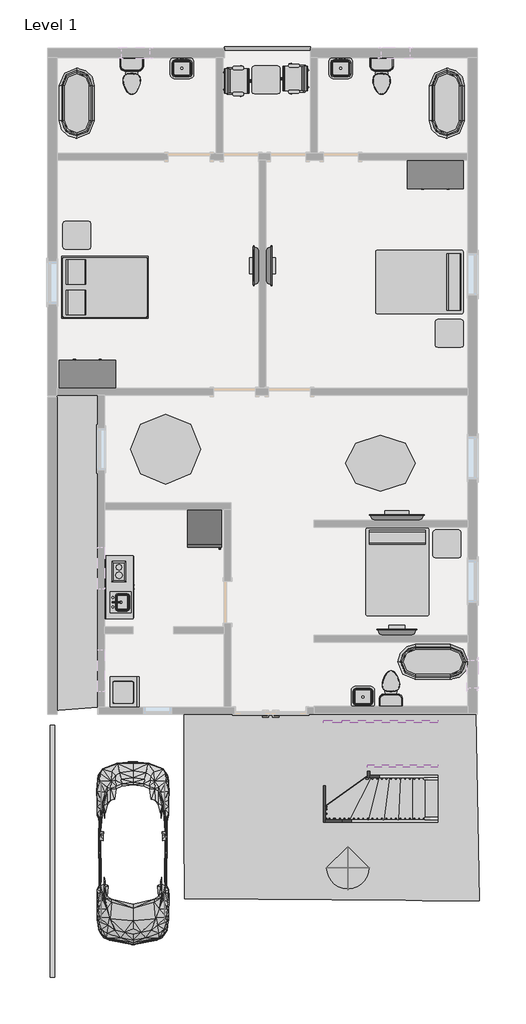
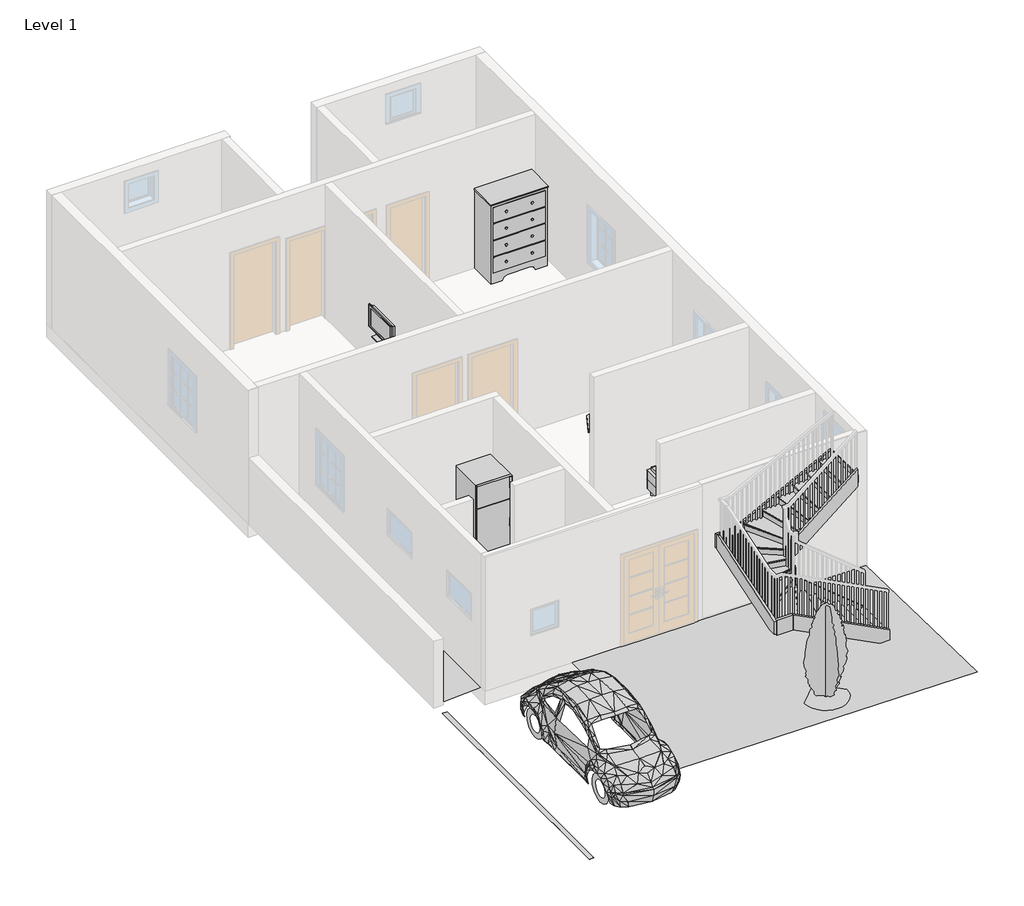
# One storey, part 3 of 3: 18 furniture elements, 10 flow terminals, 8 members, 8 proxies, 1 geographic element, 1 railing, 1 stair flight.
"""IFC4 building model written with IfcOpenShell, lengths in millimetres."""

from ifc_helpers import new_model, si_unit, point, frame, origin, origin_with_axes, place, context, project, spatial, polyline, ellipse_curve, trimmed, outline, extrude, triangles, transform, mapped, element, save
from ifc_brep_helpers import plane_surface, extruded_surface, advanced_brep
from components import proxy_fe84b772, proxy_844211aa, parking_space_9_x_18_90_deg_b8b21359, rpc_beetle_rpc_beetle_3ce7ba48, proxy_a13a33b2, proxy_718fa39f, flow_terminal_871c2e40, flow_terminal_62a433f7, toilet_domestic_3d_toilet_domestic_3d_f7549cf7, toilet_domestic_3d_toilet_domestic_3d_183bbd19, flow_terminal_b374fae2, furniture_c8abb964, furniture_0253826f, chair_task_arms_chair_task_arms_fa5a08ef, furniture_95afb093, furniture_9fa109b2, furniture_56245f3a, furniture_d9bcc661, furniture_bbcc68ce, furniture_743965d2, furniture_bcf351fa, rpc_tree_conifer_0001_chinese_juniper_7_1b9786cd, stair_flight_62da4333

model = new_model("IFC4")

# Units and contexts
model_context = context("Model", 3, world=origin())
ifc_project = project(units=[si_unit("LENGTHUNIT", "METRE", prefix="MILLI")], contexts=[model_context])

# Site, building, storey
site = spatial("IfcSite", under=ifc_project)
building = spatial("IfcBuilding", under=site)
storey = spatial("IfcBuildingStorey", under=building, Name="Level 1", Elevation=0.0)

# Proxies
placement = place(None, origin())
element("IfcBuildingElementProxy", 1, Name="Building Element Proxy", at=placement, inside=storey, context=model_context, shape_type="Tessellation", body=[
    triangles([(-8788.6245987, -108.0463665, 0.0), (-8767.5415833, -4098.269323, 0.0), (-2526.9445953, -4159.926606, 0.0), (-2604.3049896, -82.6463725, 0.0), (-8917.3917389, -4057.5674469, 0.0), (-8941.0245987, -2597.2464088, 0.0), (-8941.0245987, -108.0463665, 0.0), (-8936.3004684, -4107.611776, 0.0)], [[8, 5, 6], [5, 8, 2], [1, 7, 6], [6, 5, 2], [3, 4, 6], [3, 2, 8], [1, 4, 7], [1, 6, 4], [6, 2, 3]], closed=False),
])
element("IfcBuildingElementProxy", 2, Name="Building Element Proxy", at=placement, inside=storey, context=model_context, shape_type="Tessellation", body=[
    triangles([(-11709.6247925, 6826.153688, 0.0), (-10820.6244049, 6826.153688, 0.0), (-10820.6244049, 44.353629, 0.0), (-11811.2244049, -31.846371, 0.0)], [[1, 4, 3], [3, 2, 1]], closed=False),
])
proxy_shape = proxy_fe84b772(model_context)
element("IfcBuildingElementProxy", 3, Name="Cook Top-2 Unit : 12\" x 18\"", ObjectType="Cook Top-2 Unit : 12\" x 18\"", at=placement, inside=storey, context=model_context, shape_type="MappedRepresentation", body=[
    mapped(proxy_shape, transform((-10287.2247577, 3033.3661295, 0.0), x_axis=(-1.0, 0.0, 0.0), y_axis=(0.0, -1.0, 0.0), z_axis=(0.0, 0.0, 1.0))),
])
proxy_2_shape = proxy_844211aa(model_context)
element("IfcBuildingElementProxy", 4, Name="Kitchenette - Small : 54\"", ObjectType="Kitchenette - Small : 54\"", at=placement, inside=storey, context=model_context, shape_type="MappedRepresentation", body=[
    mapped(proxy_2_shape, transform((-10668.2247577, 2641.503629, 0.0), x_axis=(0.0, 1.0, 0.0), y_axis=(-1.0, 0.0, 0.0), z_axis=(0.0, 0.0, 1.0))),
])
parking_space_9_x_18_90_deg_shape = parking_space_9_x_18_90_deg_b8b21359(model_context)
element("IfcBuildingElementProxy", 5, Name="Parking Space : 9' x 18' - 90 deg", ObjectType="Parking Space : 9' x 18' - 90 deg", at=placement, inside=storey, context=model_context, shape_type="MappedRepresentation", body=[
    mapped(parking_space_9_x_18_90_deg_shape, transform((-11811.2247577, -336.646371, 0.0), x_axis=(1.0, 0.0, 0.0), y_axis=(0.0, 1.0, 0.0), z_axis=(0.0, 0.0, 1.0))),
])
rpc_beetle_rpc_beetle_shape = rpc_beetle_rpc_beetle_3ce7ba48(model_context)
element("IfcBuildingElementProxy", 6, Name="RPC Beetle : RPC Beetle", ObjectType="RPC Beetle : RPC Beetle", at=placement, inside=storey, context=model_context, shape_type="MappedRepresentation", body=[
    mapped(rpc_beetle_rpc_beetle_shape, transform((-10058.6247577, -1886.046371, 0.0), x_axis=(-1.0000000000000004, 0.0, 0.0), y_axis=(0.0, -1.0000000000000004, 0.0), z_axis=(0.0, 0.0, 1.0))),
])
proxy_3_shape = proxy_a13a33b2(model_context)
element("IfcBuildingElementProxy", 7, Name="Refrigerator : 30\" x 32\" RH", ObjectType="Refrigerator : 30\" x 32\" RH", at=placement, inside=storey, context=model_context, shape_type="MappedRepresentation", body=[
    mapped(proxy_3_shape, transform((-8501.2872577, 3948.4046575, 0.0), x_axis=(1.0, 0.0, 0.0), y_axis=(0.0, 1.0, 0.0), z_axis=(0.0, 0.0, 1.0))),
])
proxy_4_shape = proxy_718fa39f(model_context)
element("IfcBuildingElementProxy", 8, Name="Washer : 27\" x 25\" x 35\"", ObjectType="Washer : 27\" x 25\" x 35\"", at=placement, inside=storey, context=model_context, shape_type="MappedRepresentation", body=[
    mapped(proxy_4_shape, transform((-10515.8247577, 793.9040642, 0.0), x_axis=(0.0, -1.0000000000000016, 0.0), y_axis=(1.0000000000000016, 0.0, 0.0), z_axis=(0.0, 0.0, 1.0))),
])

# Flow terminals
flow_terminal_shape = flow_terminal_871c2e40(model_context)
element("IfcFlowTerminal", 9, ObjectType="Sink Kitchen-Island : 18\" x 18\"", at=placement, inside=storey, context=model_context, shape_type="MappedRepresentation", body=[
    mapped(flow_terminal_shape, transform((-10322.9793566, 2314.3520934, 0.0), x_axis=(0.0, 1.0, 0.0), y_axis=(-1.0, 0.0, 0.0), z_axis=(0.0, 0.0, 1.0))),
])
flow_terminal_2_shape = flow_terminal_62a433f7(model_context)
element("IfcFlowTerminal", 10, ObjectType="Sink Vanity-Square : 20\" x 18\"", at=placement, inside=storey, context=model_context, shape_type="MappedRepresentation", body=[
    mapped(flow_terminal_2_shape, transform((-9007.5139982, 13986.6082279, 304.8), x_axis=(1.0, 0.0, 0.0), y_axis=(0.0, 1.0, 0.0), z_axis=(0.0, 0.0, 1.0))),
])
element("IfcFlowTerminal", 11, ObjectType="Sink Vanity-Square : 20\" x 18\"", at=placement, inside=storey, context=model_context, shape_type="MappedRepresentation", body=[
    mapped(flow_terminal_2_shape, transform((-5553.1139982, 13986.6082279, 304.8), x_axis=(1.0, 0.0, 0.0), y_axis=(0.0, 1.0, 0.0), z_axis=(0.0, 0.0, 1.0))),
])
element("IfcFlowTerminal", 12, ObjectType="Sink Vanity-Square : 20\" x 18\"", at=placement, inside=storey, context=model_context, shape_type="MappedRepresentation", body=[
    mapped(flow_terminal_2_shape, transform((-5039.1355171, 224.4990301, 304.8), x_axis=(-1.0, 0.0, 0.0), y_axis=(0.0, -1.0, 0.0), z_axis=(0.0, 0.0, 1.0))),
])
toilet_domestic_3d_toilet_domestic_3d_shape = toilet_domestic_3d_toilet_domestic_3d_f7549cf7(model_context)
toilet_domestic_3d_toilet_domestic_3d_2_shape = toilet_domestic_3d_toilet_domestic_3d_183bbd19(model_context)
element("IfcFlowTerminal", 13, ObjectType="Toilet-Domestic-3D : Toilet-Domestic-3D", at=placement, inside=storey, context=model_context, shape_type="MappedRepresentation", body=[
    mapped(toilet_domestic_3d_toilet_domestic_3d_shape, transform((-10084.0247577, 13672.0576017, 0.0), x_axis=(1.0, 0.0, 0.0), y_axis=(0.0, 1.0, 0.0), z_axis=(0.0, 0.0, 1.0))),
    mapped(toilet_domestic_3d_toilet_domestic_3d_2_shape, transform((-10084.0247577, 13672.0576017, 0.0), x_axis=(1.0, 0.0, 0.0), y_axis=(0.0, 1.0, 0.0), z_axis=(0.0, 0.0, 1.0))),
])
element("IfcFlowTerminal", 14, ObjectType="Toilet-Domestic-3D : Toilet-Domestic-3D", at=placement, inside=storey, context=model_context, shape_type="MappedRepresentation", body=[
    mapped(toilet_domestic_3d_toilet_domestic_3d_shape, transform((-4648.4247577, 13672.0576017, 0.0), x_axis=(1.0, 0.0, 0.0), y_axis=(0.0, 1.0, 0.0), z_axis=(0.0, 0.0, 1.0))),
    mapped(toilet_domestic_3d_toilet_domestic_3d_2_shape, transform((-4648.4247577, 13672.0576017, 0.0), x_axis=(1.0, 0.0, 0.0), y_axis=(0.0, 1.0, 0.0), z_axis=(0.0, 0.0, 1.0))),
])
element("IfcFlowTerminal", 15, ObjectType="Toilet-Domestic-3D : Toilet-Domestic-3D", at=placement, inside=storey, context=model_context, shape_type="MappedRepresentation", body=[
    mapped(toilet_domestic_3d_toilet_domestic_3d_shape, transform((-4445.2247577, 539.0496564, 0.0), x_axis=(-1.0000000000000002, 0.0, 0.0), y_axis=(0.0, -1.0000000000000002, 0.0), z_axis=(0.0, 0.0, 1.0))),
    mapped(toilet_domestic_3d_toilet_domestic_3d_2_shape, transform((-4445.2247577, 539.0496564, 0.0), x_axis=(-1.0000000000000002, 0.0, 0.0), y_axis=(0.0, -1.0000000000000002, 0.0), z_axis=(0.0, 0.0, 1.0))),
])
flow_terminal_3_shape = flow_terminal_b374fae2(model_context)
element("IfcFlowTerminal", 16, ObjectType="Tub-Free Standing-3D : 30\" x 60\"", at=placement, inside=storey, context=model_context, shape_type="MappedRepresentation", body=[
    mapped(flow_terminal_3_shape, transform((-11277.8247577, 13176.153629, 0.0), x_axis=(1.0, 0.0, 0.0), y_axis=(0.0, 1.0, 0.0), z_axis=(0.0, 0.0, 1.0))),
])
element("IfcFlowTerminal", 17, ObjectType="Tub-Free Standing-3D : 30\" x 60\"", at=placement, inside=storey, context=model_context, shape_type="MappedRepresentation", body=[
    mapped(flow_terminal_3_shape, transform((-3226.0247577, 13176.153629, 0.0), x_axis=(1.0, 0.0, 0.0), y_axis=(0.0, 1.0, 0.0), z_axis=(0.0, 0.0, 1.0))),
])
element("IfcFlowTerminal", 18, ObjectType="Tub-Free Standing-3D : 30\" x 60\"", at=placement, inside=storey, context=model_context, shape_type="MappedRepresentation", body=[
    mapped(flow_terminal_3_shape, transform((-3530.8247577, 1034.953629, 0.0), x_axis=(0.0, -1.0000000000000004, 0.0), y_axis=(1.0000000000000004, 0.0, 0.0), z_axis=(0.0, 0.0, 1.0))),
])

# Furniture
furniture_shape = furniture_c8abb964(model_context)
element("IfcFurniture", 19, ObjectType="Bed-Box : Double 53\" x 74\"", at=placement, inside=storey, context=model_context, shape_type="MappedRepresentation", body=[
    mapped(furniture_shape, transform((-10902.6542659, 8836.50117, 0.0), x_axis=(0.0, 1.0000000000000002, 0.0), y_axis=(-1.0000000000000002, 0.0, 0.0), z_axis=(0.0, 0.0, 1.0))),
])
furniture_2_shape = furniture_0253826f(model_context)
element("IfcFurniture", 20, ObjectType="Bed-Standard.0001 : Double 54\" x 75\"", at=placement, inside=storey, context=model_context, shape_type="MappedRepresentation", body=[
    mapped(furniture_2_shape, transform((-3777.3296757, 9561.4421536, 0.0), x_axis=(0.0, -1.0000000000000002, 0.0), y_axis=(1.0000000000000002, 0.0, 0.0), z_axis=(0.0, 0.0, 1.0))),
])
element("IfcFurniture", 21, ObjectType="Bed-Standard.0001 : Double 54\" x 75\"", at=placement, inside=storey, context=model_context, shape_type="MappedRepresentation", body=[
    mapped(furniture_2_shape, transform((-4577.0132823, 3036.348711, 0.0), x_axis=(1.0000000000000004, 0.0, 0.0), y_axis=(0.0, 1.0000000000000004, 0.0), z_axis=(0.0, 0.0, 1.0))),
])
chair_task_arms_chair_task_arms_shape = chair_task_arms_chair_task_arms_fa5a08ef(model_context)
element("IfcFurniture", 22, ObjectType="Chair-Task Arms : Chair-Task Arms", at=placement, inside=storey, context=model_context, shape_type="MappedRepresentation", body=[
    mapped(chair_task_arms_chair_task_arms_shape, transform((-6509.078856, 13568.5628094, 0.0), x_axis=(0.0, 1.0000000000000009, 0.0), y_axis=(-1.0000000000000009, 0.0, 0.0), z_axis=(0.0, 0.0, 1.0))),
])
element("IfcFurniture", 23, ObjectType="Chair-Task Arms : Chair-Task Arms", at=placement, inside=storey, context=model_context, shape_type="MappedRepresentation", body=[
    mapped(chair_task_arms_chair_task_arms_shape, transform((-7816.9706593, 13799.7444487, 0.0), x_axis=(0.0, -1.0000000000000004, 0.0), y_axis=(1.0000000000000004, 0.0, 0.0), z_axis=(0.0, 0.0, 1.0))),
])
furniture_3_shape = furniture_95afb093(model_context)
element("IfcFurniture", 24, ObjectType="Counter Top w Sink Hole : 24\" Depth", at=placement, inside=storey, context=model_context, shape_type="MappedRepresentation", body=[
    mapped(furniture_3_shape, transform((-10668.2247577, 3174.903629, 0.0), x_axis=(0.0, 1.0, 0.0), y_axis=(-1.0, 0.0, 0.0), z_axis=(0.0, 0.0, 1.0))),
])
furniture_4_shape = furniture_9fa109b2(model_context)
element("IfcFurniture", 25, ObjectType="Dresser : 48\" x 72\" x 24\"", at=placement, inside=storey, context=model_context, shape_type="MappedRepresentation", body=[
    mapped(furniture_4_shape, transform((-11318.4180175, 6920.1906749, 0.0), x_axis=(-1.0000000000000004, 0.0, 0.0), y_axis=(0.0, -1.0000000000000004, 0.0), z_axis=(0.0, 0.0, 1.0))),
])
element("IfcFurniture", 26, ObjectType="Dresser : 48\" x 72\" x 24\"", at=placement, inside=storey, context=model_context, shape_type="MappedRepresentation", body=[
    mapped(furniture_4_shape, transform((-3210.8314978, 11989.9165831, 0.0), x_axis=(1.0, 0.0, 0.0), y_axis=(0.0, 1.0, 0.0), z_axis=(0.0, 0.0, 1.0))),
])
furniture_5_shape = furniture_56245f3a(model_context)
element("IfcFurniture", 27, ObjectType="TV - Flat Screen : 32\"", at=placement, inside=storey, context=model_context, shape_type="MappedRepresentation", body=[
    mapped(furniture_5_shape, transform((-7373.9633813, 9641.6091149, 914.4), x_axis=(0.0, -1.0000000000000004, 0.0), y_axis=(1.0000000000000004, 0.0, 0.0), z_axis=(0.0, 0.0, 1.0))),
])
element("IfcFurniture", 28, ObjectType="TV - Flat Screen : 32\"", at=placement, inside=storey, context=model_context, shape_type="MappedRepresentation", body=[
    mapped(furniture_5_shape, transform((-7104.486134, 9649.4981432, 914.4), x_axis=(0.0, 1.0000000000000002, 0.0), y_axis=(-1.0000000000000002, 0.0, 0.0), z_axis=(0.0, 0.0, 1.0))),
])
element("IfcFurniture", 29, ObjectType="TV - Flat Screen : 32\"", at=placement, inside=storey, context=model_context, shape_type="MappedRepresentation", body=[
    mapped(furniture_5_shape, transform((-4322.1692718, 1677.6922527, 914.4), x_axis=(-1.0000000000000002, 0.0, 0.0), y_axis=(0.0, -1.0000000000000002, 0.0), z_axis=(0.0, 0.0, 1.0))),
])
furniture_6_shape = furniture_d9bcc661(model_context)
element("IfcFurniture", 30, ObjectType="TV - Flat Screen : 46\"", at=placement, inside=storey, context=model_context, shape_type="MappedRepresentation", body=[
    mapped(furniture_6_shape, transform((-4322.1692718, 4166.8922527, 914.4), x_axis=(-0.9999999999999998, 0.0, 0.0), y_axis=(0.0, -0.9999999999999998, 0.0), z_axis=(0.0, 0.0, 1.0))),
])
furniture_7_shape = furniture_bbcc68ce(model_context)
element("IfcFurniture", 31, ObjectType="Table-Dining Round w Chairs : 60\" Diameter", at=placement, inside=storey, context=model_context, shape_type="MappedRepresentation", body=[
    mapped(furniture_7_shape, transform((-9451.1067249, 5842.6323176, 0.0), x_axis=(1.0, 0.0, 0.0), y_axis=(0.0, 1.0, 0.0), z_axis=(0.0, 0.0, 1.0))),
])
furniture_8_shape = furniture_743965d2(model_context)
element("IfcFurniture", 32, ObjectType="Table-Ellipse : 60\" x 48\"", at=placement, inside=storey, context=model_context, shape_type="MappedRepresentation", body=[
    mapped(furniture_8_shape, transform((-4673.8247577, 5352.953629, 0.0), x_axis=(1.0, 0.0, 0.0), y_axis=(0.0, 1.0, 0.0), z_axis=(0.0, 0.0, 1.0))),
])
furniture_9_shape = furniture_bcf351fa(model_context)
element("IfcFurniture", 33, ObjectType="Table-End : 24\" x 24\"", at=placement, inside=storey, context=model_context, shape_type="MappedRepresentation", body=[
    mapped(furniture_9_shape, transform((-11586.358388, 10153.553629, 0.0), x_axis=(1.0, 0.0, 0.0), y_axis=(0.0, 1.0, 0.0), z_axis=(0.0, 0.0, 1.0))),
])
element("IfcFurniture", 34, ObjectType="Table-End : 24\" x 24\"", at=placement, inside=storey, context=model_context, shape_type="MappedRepresentation", body=[
    mapped(furniture_9_shape, transform((-3483.758388, 8019.953629, 0.0), x_axis=(1.0, 0.0, 0.0), y_axis=(0.0, 1.0, 0.0), z_axis=(0.0, 0.0, 1.0))),
])
element("IfcFurniture", 35, ObjectType="Table-End : 24\" x 24\"", at=placement, inside=storey, context=model_context, shape_type="MappedRepresentation", body=[
    mapped(furniture_9_shape, transform((-7471.558388, 13531.753629, 0.0), x_axis=(1.0, 0.0, 0.0), y_axis=(0.0, 1.0, 0.0), z_axis=(0.0, 0.0, 1.0))),
])
element("IfcFurniture", 36, ObjectType="Table-End : 24\" x 24\"", at=placement, inside=storey, context=model_context, shape_type="MappedRepresentation", body=[
    mapped(furniture_9_shape, transform((-3534.558388, 3447.953629, 0.0), x_axis=(1.0, 0.0, 0.0), y_axis=(0.0, 1.0, 0.0), z_axis=(0.0, 0.0, 1.0))),
])

# Geographic element
rpc_tree_conifer_0001_chinese_juniper_7_shape = rpc_tree_conifer_0001_chinese_juniper_7_1b9786cd(model_context)
element("IfcGeographicElement", 37, ObjectType="RPC Tree - Conifer.0001 : Chinese Juniper - 7'", at=placement, inside=storey, context=model_context, shape_type="MappedRepresentation", body=[
    mapped(rpc_tree_conifer_0001_chinese_juniper_7_shape, transform((-5385.2214287, -3435.446371, 0.0), x_axis=(1.0, 0.0, 0.0), y_axis=(0.0, 1.0, 0.0), z_axis=(0.0, 0.0, 1.0))),
])

# Members
element("IfcMember", 38, ObjectType="Stringer - 2\" Width", at=placement, inside=storey, context=model_context, shape_type="SweptSolid", body=[
    extrude(outline(polyline([(0.0, -3425.4930658), (229.639954, -3425.4930658), (1305.3956453, -5512.9102575), (962.500629, -5512.9102575), (0.0, -3645.2553834), (0.0, -3425.4930658)])), frame((0.0, -2444.846371, 0.0), z_axis=(0.0, 1.0, 0.0), x_axis=(0.0, 0.0, 1.0)), (0.0, 0.0, 1.0), 50.8),
])
element("IfcMember", 39, ObjectType="Stringer - 2\" Width", at=placement, inside=storey, context=model_context, shape_type="SweptSolid", body=[
    extrude(outline(polyline([(-5512.9102575, -2394.046371), (-5512.9102575, -2444.846371), (-5867.6247577, -2444.846371), (-5867.6247577, -2394.046371), (-5512.9102575, -2394.046371)])), frame((0.0, 0.0, 962.500629), z_axis=(0.0, 0.0, 1.0), x_axis=(1.0, 0.0, 0.0)), (0.0, 0.0, 1.0), 342.8950162),
])
element("IfcMember", 40, ObjectType="Stringer - 2\" Width", at=placement, inside=storey, context=model_context, shape_type="SweptSolid", body=[
    extrude(outline(polyline([(-2444.846371, 1000.5956453), (-2444.846371, 1289.0952212), (-322.8264883, 1969.9972697), (-285.846371, 1969.9972697), (-285.846371, 1638.9682298), (-2275.323888, 1000.5956453), (-2444.846371, 1000.5956453)])), frame((-5918.4247577, 0.0, 0.0), z_axis=(1.0, 0.0, 0.0), x_axis=(0.0, 1.0, 0.0)), (0.0, 0.0, 1.0), 50.8),
])
element("IfcMember", 41, ObjectType="Stringer - 2\" Width", at=placement, inside=storey, context=model_context, shape_type="SweptSolid", body=[
    extrude(outline(polyline([(-5918.4247577, -285.846371), (-5918.4247577, -235.046371), (-5512.9102575, -235.046371), (-5512.9102575, -285.846371), (-5918.4247577, -285.846371)])), frame((0.0, 0.0, 1649.8904473), z_axis=(0.0, 0.0, 1.0), x_axis=(1.0, 0.0, 0.0)), (0.0, 0.0, 1.0), 320.1068224),
])
element("IfcMember", 42, ObjectType="Stringer - 2\" Width", at=placement, inside=storey, context=model_context, shape_type="SweptSolid", body=[
    extrude(outline(polyline([(1969.9972697, -5512.9102575), (1649.8904473, -5512.9102575), (2725.6461385, -3425.4930658), (3045.7529609, -3425.4930658), (1969.9972697, -5512.9102575)])), frame((0.0, -285.846371, 0.0), z_axis=(0.0, 1.0, 0.0), x_axis=(0.0, 0.0, 1.0)), (0.0, 0.0, 1.0), 50.8),
])
element("IfcMember", 43, ObjectType="Stringer - 2\" Width", at=placement, inside=storey, context=model_context, shape_type="SweptSolid", body=[
    extrude(outline(polyline([(0.0, -3425.4930658), (176.1764461, -3425.4930658), (1380.418648, -4902.4247577), (987.1410923, -4902.4247577), (0.0, -3691.7547104), (0.0, -3425.4930658)])), frame((0.0, -1479.646371, 0.0), z_axis=(0.0, 1.0, 0.0), x_axis=(0.0, 0.0, 1.0)), (0.0, 0.0, 1.0), 50.8),
])
element("IfcMember", 44, ObjectType="Stringer - 2\" Width", at=placement, inside=storey, context=model_context, shape_type="SweptSolid", body=[
    extrude(outline(polyline([(-1479.646371, 1028.5617647), (-1479.646371, 1573.2682978), (-1273.0092535, 1926.1409689), (-1251.046371, 1926.1409689), (-1251.046371, 1360.465107), (-1445.4041537, 1028.5617647), (-1479.646371, 1028.5617647)])), frame((-4953.2247577, 0.0, 0.0), z_axis=(1.0, 0.0, 0.0), x_axis=(0.0, 1.0, 0.0)), (0.0, 0.0, 1.0), 50.8),
])
element("IfcMember", 45, ObjectType="Stringer - 2\" Width", at=placement, inside=storey, context=model_context, shape_type="SweptSolid", body=[
    extrude(outline(polyline([(1926.1409689, -4953.2247577), (1532.8634131, -4953.2247577), (2778.5262875, -3425.4930658), (3171.8038432, -3425.4930658), (1926.1409689, -4953.2247577)])), frame((0.0, -1251.046371, 0.0), z_axis=(0.0, 1.0, 0.0), x_axis=(0.0, 0.0, 1.0)), (0.0, 0.0, 1.0), 50.8),
])

# Railing
element("IfcRailing", 46, ObjectType="Glass Panel - Bottom Fill", at=placement, inside=storey, context=model_context, shape_type="SolidModel", body=[
    advanced_brep(
    [(-8064.7247577, 14408.053629, 914.4), (-8064.7247577, 14331.853629, 914.4), (-6197.8247577, 14408.053629, 914.4), (-6197.8247577, 14331.853629, 914.4)],
    [
        (0, 1, ellipse_curve(frame((-8064.7247577, 14369.953629, 914.4), z_axis=(-1.0, 0.0, 0.0), x_axis=(0.0, -1.0, 0.0)), 38.1, 28.575)),
        (1, 0, ellipse_curve(frame((-8064.7247577, 14369.953629, 914.4), z_axis=(-1.0, 0.0, 0.0), x_axis=(0.0, -1.0, 0.0)), 38.1, 28.575)),
        (2, 3, ellipse_curve(frame((-6197.8247577, 14369.953629, 914.4), z_axis=(1.0, 0.0, 0.0), x_axis=(0.0, -1.0, 0.0)), 38.1, 28.575)),
        (3, 2, ellipse_curve(frame((-6197.8247577, 14369.953629, 914.4), z_axis=(1.0, 0.0, 0.0), x_axis=(0.0, -1.0, 0.0)), 38.1, 28.575)),
        (0, 2),
        (3, 1),
    ],
    [
        plane_surface(frame((-8064.7247577, 14369.953629, 914.4), z_axis=(-1.0, 0.0, 0.0), x_axis=(0.0, 1.0, 0.0))),
        plane_surface(frame((-6197.8247577, 14369.953629, 914.4), z_axis=(1.0, 0.0, 0.0), x_axis=(0.0, 1.0, 0.0))),
        extruded_surface(trimmed(ellipse_curve(frame((-6197.8247577, 14369.953629, 914.4), z_axis=(-1.0, 0.0, 0.0), x_axis=(0.0, -1.0, 0.0)), 38.1, 28.575), [point((-6197.8247577, 14408.053629, 914.4))], [point((-6197.8247577, 14331.853629, 914.4))], True, "CARTESIAN"), (-1866.8999999999996, 0.0, 0.0), 1866.8999999999996),
        extruded_surface(trimmed(ellipse_curve(frame((-6197.8247577, 14369.953629, 914.4), z_axis=(-1.0, 0.0, 0.0), x_axis=(0.0, -1.0, 0.0)), 38.1, 28.575), [point((-6197.8247577, 14331.853629, 914.4))], [point((-6197.8247577, 14408.053629, 914.4))], True, "CARTESIAN"), (-1866.8999999999996, 0.0, 0.0), 1866.8999999999996),
    ],
    [
        (0, [[1, 2]]),
        (1, [[3, 4]]),
        (2, [[-1, 5, -4, 6]]),
        (3, [[-2, -6, -3, -5]]),
    ],
),
    extrude(outline(polyline([(-8064.7247577, 14357.253629), (-8064.7247577, 14382.653629), (-6197.8247577, 14382.653629), (-6197.8247577, 14357.253629), (-8064.7247577, 14357.253629)])), frame((0.0, 0.0, 800.1), z_axis=(0.0, 0.0, 1.0), x_axis=(1.0, 0.0, 0.0)), (0.0, 0.0, 1.0), 25.4),
    extrude(outline(polyline([(-8064.7247577, 14357.253629), (-8064.7247577, 14382.653629), (-6197.8247577, 14382.653629), (-6197.8247577, 14357.253629), (-8064.7247577, 14357.253629)])), frame((0.0, 0.0, 698.5), z_axis=(0.0, 0.0, 1.0), x_axis=(1.0, 0.0, 0.0)), (0.0, 0.0, 1.0), 25.4),
    extrude(outline(polyline([(-6324.8247577, 14344.553629), (-6324.8247577, 14395.353629), (-6312.1247577, 14395.353629), (-6312.1247577, 14344.553629), (-6324.8247577, 14344.553629)])), origin_with_axes(), (0.0, 0.0, 1.0), 885.6788223),
    extrude(outline(polyline([(-7131.2747577, 14376.488786), (-6318.4747577, 14376.488786), (-6318.4747577, 14370.138786), (-7131.2747577, 14370.138786), (-7131.2747577, 14376.488786)])), frame((0.0, 0.0, 101.6), z_axis=(0.0, 0.0, 1.0), x_axis=(1.0, 0.0, 0.0)), (0.0, 0.0, 1.0), 596.9),
    extrude(outline(polyline([(-7137.6247577, 14344.553629), (-7137.6247577, 14395.353629), (-7124.9247577, 14395.353629), (-7124.9247577, 14344.553629), (-7137.6247577, 14344.553629)])), origin_with_axes(), (0.0, 0.0, 1.0), 885.6788223),
    extrude(outline(polyline([(-7944.0747577, 14376.488786), (-7131.2747577, 14376.488786), (-7131.2747577, 14370.138786), (-7944.0747577, 14370.138786), (-7944.0747577, 14376.488786)])), frame((0.0, 0.0, 101.6), z_axis=(0.0, 0.0, 1.0), x_axis=(1.0, 0.0, 0.0)), (0.0, 0.0, 1.0), 596.9),
    extrude(outline(polyline([(-7950.4247577, 14344.553629), (-7950.4247577, 14395.353629), (-7937.7247577, 14395.353629), (-7937.7247577, 14344.553629), (-7950.4247577, 14344.553629)])), origin_with_axes(), (0.0, 0.0, 1.0), 885.6788223),
    extrude(outline(polyline([(-6210.5247577, 14360.428629), (-6210.5247577, 14379.478629), (-6191.4747577, 14379.478629), (-6191.4747577, 14360.428629), (-6210.5247577, 14360.428629)])), origin_with_axes(), (0.0, 0.0, 1.0), 885.6788223),
    extrude(outline(polyline([(-8071.0747577, 14360.428629), (-8071.0747577, 14379.478629), (-8052.0247577, 14379.478629), (-8052.0247577, 14360.428629), (-8071.0747577, 14360.428629)])), origin_with_axes(), (0.0, 0.0, 1.0), 885.6788223),
])

# Stair flight
stair_flight_shape = stair_flight_62da4333(model_context)
element("IfcStairFlight", 47, ObjectType="2\" Tread 1\" Nosing 1/4\" Riser", at=placement, inside=storey, context=model_context, shape_type="MappedRepresentation", body=[
    mapped(stair_flight_shape, transform((0.0, 0.0, 0.0), x_axis=(1.0, 0.0, 0.0), y_axis=(0.0, 1.0, 0.0), z_axis=(0.0, 0.0, 1.0))),
])

save(model, "model.ifc")

# Revit data of these elements
# Type "Cook Top-2 Unit : 12\" x 18\""
#   Assembly Code = "E1090400"
#   Counter Height = 3' - 0"
#   Depth = 1' - 6"
#   Width = 1' - 0"
#   Burner Material = Steel, Chrome Plated
#   Cooktop Material = Steel, Polished
#   Default Elevation = 0
# Type "Kitchenette - Small : 54\""
#   Assembly Code = "E1090400"
#   Width = 4' - 6"
#   Height = 2' - 10 1/2"
#   Depth = 2' - 0"
#   Toe Depth = 0' - 3"
#   Toe Height = 0' - 3 1/2"
#   Cabinet Material = Cabinets
#   Door/Drawer Material = Cabinets
#   Handle Material = Cabinets - Handles
#   Default Elevation = 0
# Type "Parking Space : 9' x 18' - 90 deg"
#   Angle = 90.00°
#   Parking Length = 18' - 0"
#   Parking Width = 9' - 0"
#   pl = 18' - 0"
#   pw = 9' - 0"
# Type "RPC Beetle : RPC Beetle"
#   built-in parameter 1005195 = "RPC-16-0U6E-L4EG-ENH1-J3KF-SVEL-0TX4-C0"
#   Height = 0
# Type "Refrigerator : 30\" x 32\" RH"
#   Label = "REF."
#   Assembly Code = "E1090400"
#   Depth = 2' - 7 3/4"
#   Handle = 2' - 3"
#   Height = 5' - 10"
#   Rear Clearance = 0' - 2"
#   Top Door Height = 1' - 8"
#   Width = 2' - 5 3/8"
#   Material = Steel, Paint Finish, Ivory, Glossy
#   Default Elevation = 0
# Type "Washer : 27\" x 25\" x 35\""
#   Label = "W"
#   Assembly Code = "E1090400"
#   Depth = 2' - 1"
#   Height = 2' - 11"
#   Width = 2' - 3"
#   Washer Material = Steel, Paint Finish, Ivory, Matte
#   Default Elevation = 0
# Type "Sink Kitchen-Island : 18\" x 18\""
#   Assembly Code = "D2010410"
#   Counter Height = 3' - 0"
#   Depth = 1' - 6"
#   Width = 1' - 6"
#   Faucet Material = Steel, Polished
#   Sink Material = Steel, Polished
#   Default Elevation = 0
# Type "Sink Vanity-Square : 20\" x 18\""
#   Assembly Code = "D2010400"
#   Counter Height = 2' - 7"
#   Depth = 1' - 6"
#   Width = 1' - 8"
#   Basin Material = Porcelain, Linen
#   Faucet Material = Steel, Polished
#   Default Elevation = 0
# Type "Toilet-Domestic-3D : Toilet-Domestic-3D"
#   Assembly Code = "D2010110"
#   Toilet - Bowl/Basin Material = Porcelain, Linen
#   Toilet - Seat Material = Laminate, Linen, Matte
#   Default Elevation = 0
# Type "Tub-Free Standing-3D : 30\" x 60\""
#   Assembly Code = "D2010110"
#   Height = 1' - 6"
#   Length = 5' - 0"
#   Width = 2' - 6"
#   Tub Material = Porcelain, Ivory
#   Default Elevation = 0
# Type "Bed-Box : Double 53\" x 74\""
#   Assembly Code = "E2020200"
#   Length = 6' - 2"
#   Width = 4' - 5"
#   Frame Material = Birch
#   Mattress Material = Linen, White
#   Default Elevation = 0
# Type "Bed-Standard.0001 : Double 54\" x 75\""
#   Assembly Code = "E2020200"
#   Length = 6' - 3"
#   Width = 4' - 6"
#   Leg Material = Steel, Chrome Plated
#   Mattress Material = Linen, White
#   Default Elevation = 0
# Type "Chair-Task Arms : Chair-Task Arms"
#   Assembly Code = "E2020200"
#   Base Material = Plastic, Opaque Black
#   Caster Material = Plastic, Opaque Black
#   Seat/Back Material = Textile - Slate Blue
#   Default Elevation = 0
# Type "Counter Top w Sink Hole : 24\" Depth"
#   Assembly Code = "C1030400"
#   Counter Thickness = 0' - 1 1/2"
#   Depth [instance default] = 2' - 1"
#   Height = 3' - 0"
#   Length [instance default] = 8' - 0"
#   Sink Location [instance default] = 2' - 0"
#   Sink Location To Wall [instance default] = 0' - 6"
#   Sink Opening Depth [instance default] = 1' - 3"
#   Sink Opening Width [instance default] = 2' - 3"
#   Counter Top Material = none
#   Default Elevation = 0
# Type "Dresser : 48\" x 72\" x 24\""
#   Assembly Code = "E2020200"
#   Depth = 2' - 0"
#   Height = 6' - 0"
#   Width = 4' - 0"
#   Dresser Material = Laminate - Ivory, Glossy
#   Drawer Material = Laminate, Ivory, Matte
#   Knob Material = Cherry
#   Default Elevation = 0
# Type "TV - Flat Screen : 32\""
#   SinAng = 0' - 0.0193"
#   L = 2' - 3.79372"
#   H = 1' - 3.6354"
#   Thickness = 0' - 4.33071"
#   Diagonal = 2' - 7.88976"
#   CosAng = 0' - 0.03431"
#   Stand [instance default] = yes
#   Default Elevation = 0
# Type "TV - Flat Screen : 46\""
#   SinAng = 0' - 0.0193"
#   L = 3' - 4.83276"
#   H = 1' - 10.97053"
#   Thickness = 0' - 4.33071"
#   Diagonal = 3' - 10.85039"
#   CosAng = 0' - 0.03431"
#   Stand [instance default] = yes
#   Default Elevation = 0
# Type "Table-Dining Round w Chairs : 60\" Diameter"
#   Assembly Code = "E2020200"
#   Radius = 2' - 6"
#   Diameter = 5' - 0"
#   Height = 2' - 6"
#   Chairs = 6
#   Base Material = Pine
#   Top Material = Laminate, Linen, Matte
#   Default Elevation = 0
# Type "Table-Ellipse : 60\" x 48\""
#   Assembly Code = "E2020200"
#   Half Width = 2' - 0"
#   Half Length = 2' - 6"
#   Height = 2' - 6"
#   Length = 5' - 0"
#   Width = 4' - 0"
#   Base Material = Birch
#   Top Material = Birch
#   Default Elevation = 0
# Type "Table-End : 24\" x 24\""
#   Assembly Code = "E2020200"
#   Height = 2' - 6"
#   Length = 2' - 0"
#   Width = 2' - 0"
#   Base Material = Birch
#   Top Material = Laminate, Ivory, Matte
#   Default Elevation = 0
# Type "RPC Tree - Conifer.0001 : Chinese Juniper - 7'"
#   built-in parameter 1005198 = "{2, 15},{39, RPC-16-FUM3-UUQ0-UBF0-N000-ST1L-LVER-AU},{1, 0},{1, 0},{2, 13},{1, 8},{5, Color},{1, 0},{1, 0},{3, 0.8},{3, 0.8},{3, 0.8},{1, 8},{7, BBoxMin},{1, 0},{1, 0},{1, 0},{1, 0},{1, 0},{1, 8},{7, BBoxMax},{1, 0},{1, 0},{1, 0},{1, 0},{1, 0},{2, 11},{9, RPCTypeId},{1, 0},{1, 0},{39, RPC-16-FUM3-UUQ0-UBF0-N000-ST1L-LVER-AU},{1, 6},{14, RPCPlantHeight},{1, 0},{1, 0},{1, 7},{2, 11},{7, keyword},{1, 0},{1, 0},{34, :RPCs:Trees [General]:Geometry:RPC},{2, 11},{8, category},{1, 0},{1, 0},{15, Trees [General]},{2, 11},{12, LocalizedUID},{1, 0},{1, 0},{15, Chinese Juniper},{2, 14},{6, Height},{1, 0},{1, 0},{1, 7},{1, 2},{16, Cast Reflections},{1, 0},{1, 0},{1, 0},{1, 2},{12, Cast Shadows},{1, 0},{1, 0},{1, 1},{1, 2},{9, Lock View},{1, 0},{1, 0},{1, 0},{1, 4},{5, ViewC},{1, 0},{1, 0},{1, 0},{21, assetlibrary_base.fbx},{1, 5},"
#   built-in parameter 1005195 = "RPC-16-FUM3-UUQ0-UBF0-N000-ST1L-LVER-AU"
#   Type Comments = "Chinese Juniper"
#   Assembly Code = "G2050500"
#   Height = 7' - 0"
#   Description = (empty or 0)
#   Default Elevation = 0
# Type "Glass Panel - Bottom Fill"
#   Assembly Code = "C2010400"
#   built-in parameter 1008612 = 0.0416667 (stored number, unit not read)
#   built-in parameter 1008611 = 0.0416667 (stored number, unit not read)
#   built-in parameter 1008609 = 0.333333 (stored number, unit not read)
#   built-in parameter 1008604 = 0.166667 (stored number, unit not read)
#   built-in parameter 1008603 = 0.166667 (stored number, unit not read)
#   Railing Height = 3' - 0"
#   built-in parameter 1008630 = 2
#   built-in parameter 1008610 = 2
#   built-in parameter 1008618 = Baluster - Square : 3/4"
# Elements 1, 2 (IfcBuildingElementProxy)
#   Material = none
#   Phase Created = New Construction
# Element 3 (IfcBuildingElementProxy, "Cook Top-2 Unit : 12\" x 18\"")
#   Phase Created = New Construction
#   Materials on its faces: "Steel, Chrome Plated", "Steel, Polished"
# Element 4 (IfcBuildingElementProxy, "Kitchenette - Small : 54\"")
#   Phase Created = New Construction
#   Materials on its faces: "Cabinets", "Cabinets - Handles"
# Element 5 (IfcBuildingElementProxy, "Parking Space : 9' x 18' - 90 deg")
#   Phase Created = New Construction
#   Materials on its faces: "Parking Stripe"
# Element 6 (IfcBuildingElementProxy, "RPC Beetle : RPC Beetle")
#   Phase Created = New Construction
# Element 7 (IfcBuildingElementProxy, "Refrigerator : 30\" x 32\" RH")
#   Phase Created = New Construction
#   Materials on its faces: "Steel, Paint Finish, Ivory, Glossy", "Steel, Chrome Plated"
# Element 8 (IfcBuildingElementProxy, "Washer : 27\" x 25\" x 35\"")
#   Phase Created = New Construction
#   Materials on its faces: "Steel, Paint Finish, Ivory, Matte"
# Element 9 (IfcFlowTerminal, "Sink Kitchen-Island : 18\" x 18\"")
#   Mark = "7"
#   Phase Created = New Construction
#   Materials on its faces: "Steel, Polished"
# Element 10 (IfcFlowTerminal, "Sink Vanity-Square : 20\" x 18\"")
#   Mark = "3"
#   Phase Created = New Construction
#   Materials on its faces: "Porcelain, Linen", "Steel, Polished"
# Element 11 (IfcFlowTerminal, "Sink Vanity-Square : 20\" x 18\"")
#   Mark = "5"
#   Phase Created = New Construction
#   Materials on its faces: "Porcelain, Linen", "Steel, Polished"
# Element 12 (IfcFlowTerminal, "Sink Vanity-Square : 20\" x 18\"")
#   Mark = "10"
#   Phase Created = New Construction
#   Materials on its faces: "Porcelain, Linen", "Steel, Polished"
# Element 13 (IfcFlowTerminal, "Toilet-Domestic-3D : Toilet-Domestic-3D")
#   Mark = "2"
#   Phase Created = New Construction
#   Materials on its faces: "Porcelain, Linen", "Laminate, Linen, Matte"
# Element 14 (IfcFlowTerminal, "Toilet-Domestic-3D : Toilet-Domestic-3D")
#   Mark = "4"
#   Phase Created = New Construction
#   Materials on its faces: "Porcelain, Linen", "Laminate, Linen, Matte"
# Element 15 (IfcFlowTerminal, "Toilet-Domestic-3D : Toilet-Domestic-3D")
#   Mark = "9"
#   Phase Created = New Construction
#   Materials on its faces: "Porcelain, Linen", "Laminate, Linen, Matte"
# Element 16 (IfcFlowTerminal, "Tub-Free Standing-3D : 30\" x 60\"")
#   Mark = "1"
#   Phase Created = New Construction
#   Materials on its faces: "Porcelain, Ivory"
# Element 17 (IfcFlowTerminal, "Tub-Free Standing-3D : 30\" x 60\"")
#   Mark = "6"
#   Phase Created = New Construction
#   Materials on its faces: "Porcelain, Ivory"
# Element 18 (IfcFlowTerminal, "Tub-Free Standing-3D : 30\" x 60\"")
#   Mark = "8"
#   Phase Created = New Construction
#   Materials on its faces: "Porcelain, Ivory"
# Element 19 (IfcFurniture, "Bed-Box : Double 53\" x 74\"")
#   Phase Created = New Construction
#   Materials on its faces: "Birch", "Linen, White"
# Elements 20, 21 (IfcFurniture, "Bed-Standard.0001 : Double 54\" x 75\"")
#   Phase Created = New Construction
#   Materials on its faces: "Linen, White", "Steel, Chrome Plated"
# Elements 22, 23 (IfcFurniture, "Chair-Task Arms : Chair-Task Arms")
#   Phase Created = New Construction
#   Materials on its faces: "Plastic, Opaque Black", "Textile - Slate Blue"
# Element 24 (IfcFurniture, "Counter Top w Sink Hole : 24\" Depth")
#   Sink Opening Depth = 1' - 3"
#   Sink Location To Wall = 0' - 6"
#   Length = 4' - 6"
#   Sink Location = 1' - 2"
#   Sink Opening Width = 1' - 4"
#   Depth = 2' - 0"
#   Phase Created = New Construction
#   Materials on its faces: "Counter Top"
# Elements 25, 26 (IfcFurniture, "Dresser : 48\" x 72\" x 24\"")
#   Phase Created = New Construction
#   Materials on its faces: "Laminate, Ivory, Matte", "Cherry", "Laminate - Ivory, Glossy"
# Elements 27, 28, 29 (IfcFurniture, "TV - Flat Screen : 32\"")
#   Stand = yes
#   Phase Created = New Construction
#   Materials on its faces: "TV - Black", "TV - Glass", "TV - Screen"
# Element 30 (IfcFurniture, "TV - Flat Screen : 46\"")
#   Stand = yes
#   Phase Created = New Construction
#   Materials on its faces: "TV - Black", "TV - Glass", "TV - Screen"
# Element 31 (IfcFurniture, "Table-Dining Round w Chairs : 60\" Diameter")
#   Phase Created = New Construction
#   Materials on its faces: "Pine", "Laminate, Linen, Matte"
# Element 32 (IfcFurniture, "Table-Ellipse : 60\" x 48\"")
#   Phase Created = New Construction
#   Materials on its faces: "Birch"
# Elements 33, 34, 35, 36 (IfcFurniture, "Table-End : 24\" x 24\"")
#   Phase Created = New Construction
#   Materials on its faces: "Laminate, Ivory, Matte", "Birch"
# Element 37 (IfcGeographicElement, "RPC Tree - Conifer.0001 : Chinese Juniper - 7'")
#   Phase Created = New Construction
# Elements 38, 39, 40, 41, 42, 43, 44, 45 (IfcMember, "Stringer - 2\" Width")
#   Phase Created = New Construction
# Element 46 (IfcRailing, "Glass Panel - Bottom Fill")
#   Phase Created = New Construction
#   Materials on its faces: "Glass"
# Element 47 (IfcStairFlight, "2\" Tread 1\" Nosing 1/4\" Riser")
#   Phase Created = New Construction
# Materials
#   "Steel, Chrome Plated": class "Metal", colour RGB 17 17 17, transparency 0, Description = "Chromiuim plated steel", Cost = 0
#   "Steel, Polished": class "Metal", colour RGB 57 57 57, transparency 0, Description = "Polished steel", Cost = 0
#   "Cabinets": colour RGB 249 249 249, transparency 0
#   "Cabinets - Handles": class "Metal", colour RGB 57 57 57, transparency 0
#   "Steel, Paint Finish, Ivory, Glossy": class "Metal", colour RGB 247 247 239, transparency 0, Description = "Steel, paint finish, ivory, glossy", Cost = 0
#   "Steel, Paint Finish, Ivory, Matte": class "Metal", colour RGB 247 247 239, transparency 0, Description = "Steel, paint finish, ivory, matte", Cost = 0
#   "Porcelain, Linen": class "Ceramic", colour RGB 249 239 230, transparency 0, Description = "Porcelain, linen", Cost = 0
#   "Laminate, Linen, Matte": class "Plastic", colour RGB 249 239 230, transparency 0, Description = "Plastic Laminate - Linen, Matte", Cost = 0
#   "Porcelain, Ivory": class "Ceramic", colour RGB 247 247 239, transparency 0, Description = "Porcelain, ivory", Cost = 0
#   "Birch": class "Wood", colour RGB 224 178 126, transparency 0, Description = "Betula Alleghaniensis", Cost = 0
#   "Linen, White": class "Textile", colour RGB 247 247 239, transparency 0, Description = "Linen, white", Cost = 0
#   "Plastic, Opaque Black": class "Plastic", colour RGB 0 0 0, transparency 0.7, Description = "Plastic, generic, opaque black", Cost = 0
#   "Textile - Slate Blue": class "Fabric", colour RGB 98 102 118, transparency 0
#   "Laminate - Ivory, Glossy": colour RGB 247 247 239, transparency 0
#   "Laminate, Ivory, Matte": class "Plastic", colour RGB 247 247 239, transparency 0, Description = "Plastic Laminate - Ivory, Matte", Cost = 0
#   "Cherry": class "Wood", colour RGB 226 177 128, transparency 0, Description = "Prunus Serotina", Cost = 0
#   "Pine": class "Wood", colour RGB 223 192 134, transparency 0, Description = "Pinus Echinata", Cost = 0
#   "Parking Stripe": class "Paint", colour RGB 250 250 91, transparency 0
#   "Counter Top": class "Wood", colour RGB 226 177 128, transparency 0
#   "TV - Black": colour RGB 49 49 49, transparency 0
#   "TV - Glass": colour RGB 157 157 157, transparency 0.9
#   "TV - Screen": colour RGB 0 0 0, transparency 0
#   "Glass": class "Glass", colour RGB 0 128 192, transparency 0.75, Description = "Soda Lime Glass", Cost = 0
